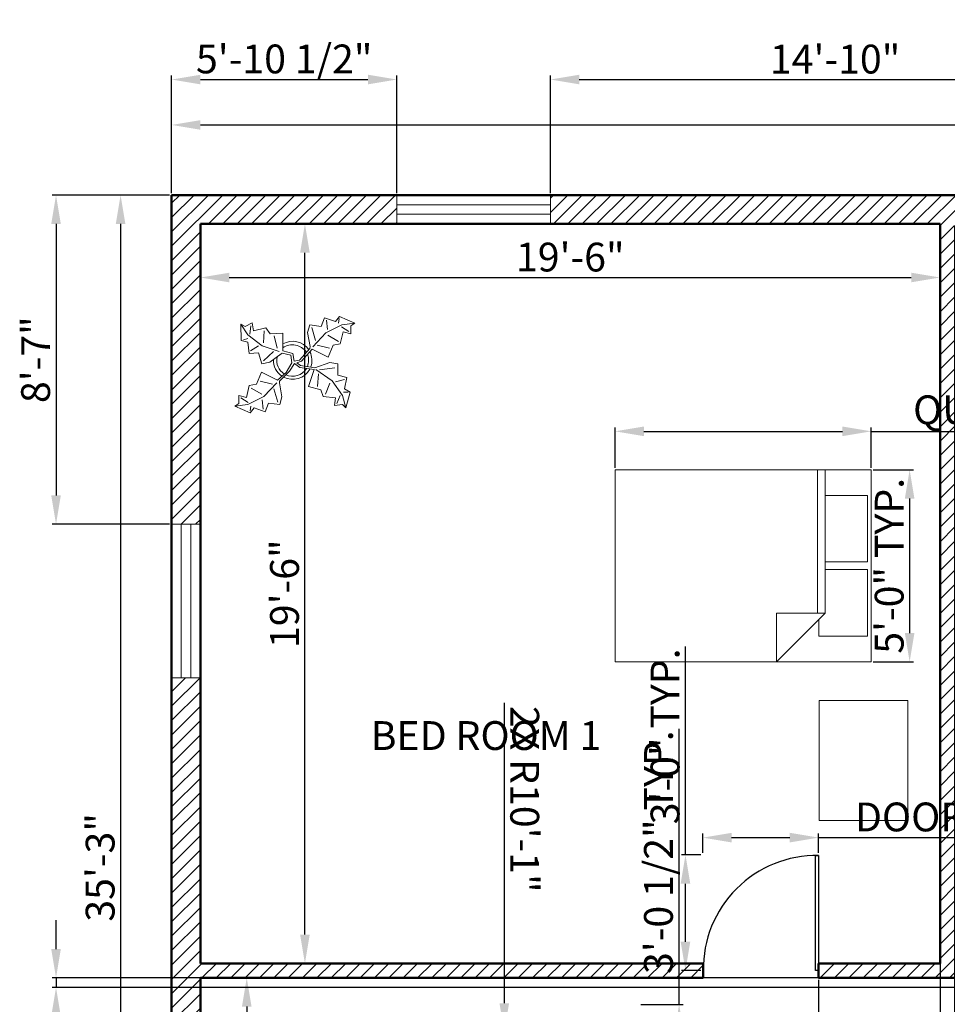
# Model space of a CAD drawing. Units: inches. Extents: x 61993 to 62774, y 55335 to 55871.
# Tile 3 of 6: x 62021 to 62310, y 55563 to 55871. Entities that reach past the tile are written whole.
import ezdxf

# ---------------------------------------------------------------- set-up
doc = ezdxf.new("R2010")
doc.units = ezdxf.units.IN
for name, color, linetype, lineweight in [('A-ANNO-DIMS', 2, 'Continuous', 18), ('A-AREA-IDEN', 7, 'Continuous', 25), ('A-DOOR', 3, 'Continuous', 25), ('A-FURN', 9, 'Continuous', 18), ('A-FURN-PLNT', 94, 'Continuous', 13), ('A-GLAZ', 4, 'Continuous', 18), ('A-WALL', 7, 'Continuous', 50)]:
    doc.layers.add(name, color=color, linetype=linetype, lineweight=lineweight)
doc.layers.add('A-WALL-PATT', color=40, linetype='Continuous', lineweight=13, true_color=0xf8d731)
doc.styles.get("Standard").update_dxf_attribs({"font": 'arial.ttf'})
doc.dimstyles.new('ISO-25', dxfattribs={"dimtxt": 9, "dimasz": 9, "dimexe": 1.25, "dimexo": 0.625, "dimtad": 1, "dimdec": 1, "dimrnd": 9, "dimlunit": 3, "dimtxsty": 'Standard', "dimcen": 2.5, "dimadec": 0, "dimazin": 0, "dimtfac": 1, "dimtdec": 1, "dimtmove": 0, "dimatfit": 3, "dimfxl": 1, "dimarcsym": 0})

# ---------------------------------------------------------------- blocks, each defined once
blk = doc.blocks.new('*D1')
at = {"layer": 'A-ANNO-DIMS', "color": 0, "lineweight": -2, "transparency": 16777216}
for p, q in [((62077.82, 55806.96), (62111.07, 55806.96)), ((62109.82, 55584.96), (62109.82, 55797.96)), ((62077.82, 55575.96), (62111.07, 55575.96))]:
    blk.add_line(p, q, dxfattribs=at)
at = {"layer": 'A-ANNO-DIMS', "color": 0, "transparency": 16777216}
for points in [[(62108.32, 55797.96), (62111.32, 55797.96), (62109.82, 55806.96)], [(62108.32, 55584.96), (62111.32, 55584.96), (62109.82, 55575.96)]]:
    blk.add_solid(points, dxfattribs=at)
at = {"layer": 'Defpoints', "color": 0, "transparency": 16777216}
for p in [(62077.19, 55806.96), (62109.82, 55806.96), (62077.19, 55575.96)]:
    blk.add_point(p, dxfattribs=at)
at = {"layer": 'A-ANNO-DIMS', "color": 0, "transparency": 16777216, "insert": (62104.6, 55691.46), "char_height": 9, "attachment_point": 5, "rotation": 90}
blk.add_mtext('19\'-6"', dxfattribs=at)
blk = doc.blocks.new('*D2')
at = {"layer": 'A-ANNO-DIMS', "color": 0, "lineweight": -2, "transparency": 16777216}
for p, q in [((62077.19, 55806.33), (62077.19, 55788.97)), ((62308.19, 55806.33), (62308.19, 55788.97)), ((62086.19, 55790.22), (62299.19, 55790.22))]:
    blk.add_line(p, q, dxfattribs=at)
at = {"layer": 'A-ANNO-DIMS', "color": 0, "transparency": 16777216}
for points in [[(62086.19, 55791.72), (62086.19, 55788.72), (62077.19, 55790.22)], [(62299.19, 55791.72), (62299.19, 55788.72), (62308.19, 55790.22)]]:
    blk.add_solid(points, dxfattribs=at)
at = {"layer": 'Defpoints', "color": 0, "transparency": 16777216}
for p in [(62077.19, 55806.96), (62308.19, 55806.96), (62308.19, 55790.22)]:
    blk.add_point(p, dxfattribs=at)
at = {"layer": 'A-ANNO-DIMS', "color": 0, "transparency": 16777216, "insert": (62192.69, 55795.44), "char_height": 9, "attachment_point": 5}
blk.add_mtext('19\'-6"', dxfattribs=at)
blk = doc.blocks.new('*D11')
at = {"layer": 'A-ANNO-DIMS', "color": 0, "lineweight": -2, "transparency": 16777216}
for p, q in [((62077.82, 55571.46), (62092.9, 55571.46)), ((62091.65, 55562.46), (62091.65, 55413.96)), ((62077.82, 55404.96), (62092.9, 55404.96))]:
    blk.add_line(p, q, dxfattribs=at)
at = {"layer": 'A-ANNO-DIMS', "color": 0, "transparency": 16777216}
for points in [[(62090.15, 55562.46), (62093.15, 55562.46), (62091.65, 55571.46)], [(62090.15, 55413.96), (62093.15, 55413.96), (62091.65, 55404.96)]]:
    blk.add_solid(points, dxfattribs=at)
at = {"layer": 'Defpoints', "color": 0, "transparency": 16777216}
for p in [(62077.19, 55571.46), (62077.19, 55404.96), (62091.65, 55404.96)]:
    blk.add_point(p, dxfattribs=at)
at = {"layer": 'A-ANNO-DIMS', "color": 0, "transparency": 16777216, "insert": (62086.43, 55488.21), "char_height": 9, "attachment_point": 5, "rotation": 90}
blk.add_mtext('14\'-3"', dxfattribs=at)
blk = doc.blocks.new('Bed - Queen')
for p, q in [((0, -80.00003), (0, 0)), ((0, 0), (59.99999, 0)), ((59.99999, 0), (59.99999, -80.00003)), ((7.99999, -1.2), (28.79998, -1.2)), ((7.99999, -14.4), (7.99999, -1.2)), ((28.79998, -1.2), (28.79998, -14.4)), ((31.19999, -1.2), (51.99999, -1.2)), ((31.19999, -14.4), (31.19999, -1.2)), ((51.99999, -1.2), (51.99999, -16.4)), ((0, -14.4), (44.8, -14.4)), ((59.99999, -29.6), (44.8, -14.4)), ((44.8, -14.4), (44.8, -29.6)), ((44.8, -16.8), (0, -16.8)), ((51.99999, -16.4), (46.79936, -16.4)), ((44.8, -29.6), (59.99999, -29.6)), ((59.99999, -80.00003), (0, -80.00003))]:
    blk.add_line(p, q)
blk = doc.blocks.new('Plant - Rubber or Philodendron')
for p, q in [((8.8871, 10.7908), (9.9809, 13.4933)), ((9.9809, 13.4933), (13.3837, 12.301)), ((10.5828, 12.6946), (10.8893, 9.7953)), ((13.3837, 12.301), (14.68, 13.9039)), ((14.5816, 13.2037), (14.3848, 11.8033)), ((14.68, 13.9039), (19.3848, 11.8146)), ((-16.2005, 11.4774), (-13.9899, 8.1064)), ((-16.2005, 11.4774), (-14.8639, 10.7964)), ((-16.0159, 6.3329), (-16.2005, 11.4774)), ((-14.8639, 10.7964), (-12.6195, 11.8975)), ((-13.3174, 8.325), (-13.0735, 11.0065)), ((-12.6195, 11.8975), (-12.1909, 9.4345)), ((-12.1909, 9.4345), (-8.3829, 10.3)), ((-8.8369, 9.409), (-9.0894, 5.6095)), ((-8.3829, 10.3), (-7.0549, 8.501)), ((4.6914, 8.8812), (5.3859, 11.2828)), ((5.3859, 11.2828), (8.8871, 10.7908)), ((5.9878, 10.4842), (7.1971, 6.3869)), ((15.3859, 11.3055), (10.3916, 8.7942)), ((15.2875, 10.6053), (17.5907, 9.2105)), ((19.3848, 11.8146), (15.3859, 11.3055)), ((19.3848, 11.8146), (18.1868, 10.9119)), ((18.1868, 10.9119), (18.1925, 8.4119)), ((-14.0069, 5.8704), (-16.0159, 6.3329)), ((-15.3434, 6.5514), (-13.9984, 6.9884)), ((-13.9899, 8.1064), (-9.5434, 4.7185)), ((-7.0549, 8.501), (-3.0284, 8.6941)), ((-4.8529, 4.012), (-5.7184, 7.82)), ((-3.0284, 8.6941), (-3.0709, 3.1041)), ((4.6914, 8.8812), (5.5014, 4.4831)), ((10.3916, 8.7942), (6.2847, 4.4028)), ((14.2977, 6.1031), (10.9934, 7.9956)), ((15.7909, 9.1065), (14.8995, 5.3044)), ((18.1925, 8.4119), (15.7909, 9.1065)), ((-13.5868, 2.2894), (-14.0069, 5.8704)), ((-13.1329, 3.1804), (-10.6614, 4.727)), ((-9.5434, 4.7185), (-4.1917, 2.9888)), ((-3.0709, 3.1041), (0.0797, 2.3163)), ((2.1141, 0.2298), (5.4346, 3.9146)), ((6.1032, 3.6844), (2.8262, -0.031)), ((5.4346, 3.9146), (5.5014, 4.4831)), ((11.1089, 1.1958), (6.1032, 3.6844)), ((7.7005, 4.8881), (11.5025, 3.9967)), ((12.7005, 4.8994), (11.1089, 1.1958)), ((14.8995, 5.3044), (12.7005, 4.8994)), ((-10.6784, 2.491), (-13.5868, 2.2894)), ((-9.5858, -0.8715), (-10.6784, 2.491)), ((-9.1318, 0.0195), (-5.9793, 2.9025)), ((-7.1228, -0.443), (-3.5248, 2.2131)), ((-3.5248, 2.2131), (-3.3011, 2.4355)), ((-3.3011, 2.4355), (-0.5306, 1.7947)), ((-0.5306, 1.7947), (-0.2255, -0.5527)), ((-0.5306, 1.7947), (-0.5306, 1.7947)), ((0.0797, 2.3163), (0.4866, -0.031)), ((0.4866, -0.031), (2.1141, 0.2298)), ((-7.1228, -0.443), (-9.5858, -0.8715)), ((-2.019, -3.6148), (-0.2255, -0.5527)), ((-0.9375, -3.1608), (0.5883, -0.8135)), ((0.5883, -0.8135), (2.2447, -2.0916)), ((2.8262, -0.031), (1.3003, -0.5527)), ((1.3003, -0.5527), (2.4193, -1.4655)), ((2.2447, -2.0916), (6.7108, -2.6626)), ((2.4193, -1.4655), (6.895, -2.1175)), ((4.943, -7.9659), (6.7108, -2.6626)), ((11.6605, -0.5413), (6.895, -2.1175)), ((12.3677, -6.1981), (7.219, -2.6772)), ((8.3544, -2.7453), (13.1973, -2.1704)), ((11.6605, -0.5413), (14.1354, -0.8948)), ((14.1354, -0.8948), (14.1354, -4.4304)), ((-11.3237, -7.2629), (-9.7321, -3.5593)), ((-9.7321, -3.5593), (-4.7264, -6.0479)), ((-2.019, -3.6148), (-4.7264, -6.0479)), ((-4.0579, -6.2781), (-0.9375, -3.1608)), ((8.125, -4.0768), (7.7715, -7.9659)), ((16.2567, -5.8446), (13.4283, -6.5517)), ((14.1354, -4.4304), (16.9638, -5.1375)), ((16.9638, -5.1375), (16.2567, -8.673)), ((-14.4141, -11.4699), (-13.5228, -7.6679)), ((-13.5228, -7.6679), (-11.3237, -7.2629)), ((-12.921, -8.4665), (-9.6166, -10.359)), ((-6.3237, -7.2516), (-10.1257, -6.3602)), ((-9.0148, -11.1577), (-4.9047, -6.8122)), ((-4.611, -12.8477), (-5.8203, -8.7504)), ((-4.1246, -6.8466), (-4.0579, -6.2781)), ((-3.3146, -11.2447), (-4.1246, -6.8466)), ((8.8321, -9.0266), (4.943, -7.9659)), ((9.5392, -11.1479), (8.8321, -9.0266)), ((10.2463, -10.4408), (11.6605, -6.9053)), ((15.5496, -10.7943), (12.3677, -6.1981)), ((16.2567, -8.673), (18.0245, -9.7337)), ((-16.8157, -10.7754), (-14.4141, -11.4699)), ((-16.8101, -13.2754), (-16.8157, -10.7754)), ((-13.9107, -12.9688), (-16.2139, -11.574)), ((-14.0091, -13.669), (-9.0148, -11.1577)), ((-9.206, -15.0581), (-9.5126, -12.1588)), ((-3.3146, -11.2447), (-4.0092, -13.6463)), ((13.4283, -11.5015), (9.5392, -11.1479)), ((13.0748, -13.9763), (13.4283, -11.5015)), ((14.8425, -10.7943), (13.7819, -13.2692)), ((16.6103, -14.6834), (15.5496, -10.7943)), ((17.3174, -9.7337), (15.9032, -9.7337)), ((18.0245, -9.7337), (16.6103, -14.6834)), ((-18.008, -14.1781), (-16.8101, -13.2754)), ((-18.008, -14.1781), (-14.0091, -13.669)), ((-13.3032, -16.2674), (-18.008, -14.1781)), ((-12.0069, -14.6645), (-13.3032, -16.2674)), ((-13.2048, -15.5672), (-13.008, -14.1668)), ((-8.6042, -15.8568), (-12.0069, -14.6645)), ((-7.5103, -13.1543), (-8.6042, -15.8568)), ((-4.0092, -13.6463), (-7.5103, -13.1543)), ((15.5496, -13.6228), (13.0748, -13.9763)), ((16.6103, -14.6834), (15.5496, -13.6228))]:
    blk.add_line(p, q)
for centre, radius, start, end in [((0, 0), 6.1275, 34.37569, 120.1028), ((-0.0601, -0.2075), 5.2461, 33.82192, 124.9414), ((0.0308, 0.1664), 6, 178.6147, 235.1169), ((0.0308, 0.1664), 5, 168.1647, 238.6725), ((-0.2664, 0.1682), 5.2775, 338.4094, 20.03007), ((-0.098, 0.1364), 6.1288, 341.2017, 26.09184), ((-0.0234, 0.3825), 6.1492, 242.5812, 331.2714), ((-0.1102, 0.4886), 5.2883, 247.3711, 327.472)]:
    blk.add_arc(centre, radius, start, end)
blk = doc.blocks.new('*D24')
at = {"layer": 'A-ANNO-DIMS', "color": 0, "lineweight": -2, "transparency": 16777216}
for p, q in [((62068.19, 55816.58), (62068.19, 55839.13)), ((62728.19, 55816.58), (62728.19, 55839.13)), ((62077.19, 55837.88), (62719.19, 55837.88))]:
    blk.add_line(p, q, dxfattribs=at)
at = {"layer": 'A-ANNO-DIMS', "color": 0, "transparency": 16777216}
for points in [[(62077.19, 55839.38), (62077.19, 55836.38), (62068.19, 55837.88)], [(62719.19, 55839.38), (62719.19, 55836.38), (62728.19, 55837.88)]]:
    blk.add_solid(points, dxfattribs=at)
at = {"layer": 'Defpoints', "color": 0, "transparency": 16777216}
for p in [(62728.19, 55837.88), (62068.19, 55815.96), (62728.19, 55815.96)]:
    blk.add_point(p, dxfattribs=at)
at = {"layer": 'A-ANNO-DIMS', "color": 0, "transparency": 16777216, "insert": (62398.19, 55843.1), "char_height": 9, "attachment_point": 5}
blk.add_mtext('54\'-9"', dxfattribs=at)
blk = doc.blocks.new('*D27')
at = {"layer": 'A-ANNO-DIMS', "color": 0, "lineweight": -2, "transparency": 16777216}
for p, q in [((62067.57, 55815.96), (62051, 55815.96)), ((62052.25, 55806.96), (62052.25, 55404.96)), ((62067.57, 55395.96), (62051, 55395.96))]:
    blk.add_line(p, q, dxfattribs=at)
at = {"layer": 'A-ANNO-DIMS', "color": 0, "transparency": 16777216}
for points in [[(62050.75, 55806.96), (62053.75, 55806.96), (62052.25, 55815.96)], [(62050.75, 55404.96), (62053.75, 55404.96), (62052.25, 55395.96)]]:
    blk.add_solid(points, dxfattribs=at)
at = {"layer": 'Defpoints', "color": 0, "transparency": 16777216}
for p in [(62068.19, 55815.96), (62052.25, 55395.96), (62068.19, 55395.96)]:
    blk.add_point(p, dxfattribs=at)
at = {"layer": 'A-ANNO-DIMS', "color": 0, "transparency": 16777216, "insert": (62047.03, 55605.96), "char_height": 9, "attachment_point": 5, "rotation": 90}
blk.add_mtext('35\'-3"', dxfattribs=at)
blk = doc.blocks.new('WIN-48IN')
for p, q in [((0, 9), (0, 0)), ((48, 9), (48, 0)), ((48, 6), (0, 6)), ((48, 3), (0, 3))]:
    blk.add_line(p, q)
blk = doc.blocks.new('DOOR-SINGLE-36IN')
for p, q in [((35, 0), (35, 36)), ((35, 36), (36, 36)), ((36, 36), (36, 2.25)), ((36, 0), (35, 0))]:
    blk.add_line(p, q)
blk.add_arc((35.5, 0.5), 35.5, 89.1931, 180.8069)
blk = doc.blocks.new('TABLE-BEDSIDE')
blk.add_lwpolyline([(0, 37.52), (27.74, 37.52), (27.74, 0), (0, 0)], close=True)
blk = doc.blocks.new('*D34')
at = {"layer": 'A-ANNO-DIMS', "color": 0, "lineweight": -2, "transparency": 16777216}
for p, q in [((62234.09, 55610.47), (62234.09, 55616.51)), ((62243.09, 55615.26), (62261.23, 55615.26)), ((62270.23, 55610.47), (62270.23, 55616.51)), ((62270.23, 55615.26), (62376.1, 55615.26))]:
    blk.add_line(p, q, dxfattribs=at)
at = {"layer": 'A-ANNO-DIMS', "color": 0, "transparency": 16777216}
for points in [[(62243.09, 55616.76), (62243.09, 55613.76), (62234.09, 55615.26)], [(62261.23, 55616.76), (62261.23, 55613.76), (62270.23, 55615.26)]]:
    blk.add_solid(points, dxfattribs=at)
at = {"layer": 'Defpoints', "color": 0, "transparency": 16777216}
for p in [(62270.23, 55615.26), (62234.09, 55609.84), (62270.23, 55609.84)]:
    blk.add_point(p, dxfattribs=at)
at = {"layer": 'A-ANNO-DIMS', "color": 0, "transparency": 16777216, "insert": (62327.67, 55620.55), "char_height": 9, "attachment_point": 5}
blk.add_mtext('DOOR 3\'-0" TYP.', dxfattribs=at)
blk = doc.blocks.new('*D35')
at = {"layer": 'A-ANNO-DIMS', "color": 0, "lineweight": -2, "transparency": 16777216}
for p, q in [((62228.67, 55609.84), (62228.67, 55674.94)), ((62233.47, 55609.84), (62227.42, 55609.84)), ((62228.67, 55582.71), (62228.67, 55600.84)), ((62233.47, 55573.71), (62227.42, 55573.71))]:
    blk.add_line(p, q, dxfattribs=at)
at = {"layer": 'A-ANNO-DIMS', "color": 0, "transparency": 16777216}
for points in [[(62227.17, 55600.84), (62230.17, 55600.84), (62228.67, 55609.84)], [(62227.17, 55582.71), (62230.17, 55582.71), (62228.67, 55573.71)]]:
    blk.add_solid(points, dxfattribs=at)
at = {"layer": 'Defpoints', "color": 0, "transparency": 16777216}
for p in [(62228.67, 55609.84), (62234.09, 55609.84), (62234.09, 55573.71)]:
    blk.add_point(p, dxfattribs=at)
at = {"layer": 'A-ANNO-DIMS', "color": 0, "transparency": 16777216, "insert": (62223.45, 55646.89), "char_height": 9, "attachment_point": 5, "rotation": 90}
blk.add_mtext('3\'-0" TYP.', dxfattribs=at)
blk = doc.blocks.new('*D38')
at = {"layer": 'A-ANNO-DIMS', "color": 0, "lineweight": -2, "transparency": 16777216}
for p, q in [((62206.68, 55730.79), (62206.68, 55743.42)), ((62286.68, 55730.79), (62286.68, 55743.42)), ((62215.68, 55742.17), (62277.68, 55742.17)), ((62286.68, 55742.17), (62429.32, 55742.17))]:
    blk.add_line(p, q, dxfattribs=at)
at = {"layer": 'A-ANNO-DIMS', "color": 0, "transparency": 16777216}
for points in [[(62215.68, 55743.67), (62215.68, 55740.67), (62206.68, 55742.17)], [(62277.68, 55743.67), (62277.68, 55740.67), (62286.68, 55742.17)]]:
    blk.add_solid(points, dxfattribs=at)
at = {"layer": 'Defpoints', "color": 0, "transparency": 16777216}
for p in [(62286.68, 55742.17), (62206.68, 55730.17), (62286.68, 55730.17)]:
    blk.add_point(p, dxfattribs=at)
at = {"layer": 'A-ANNO-DIMS', "color": 0, "transparency": 16777216, "insert": (62362.5, 55747.72), "char_height": 9, "attachment_point": 5}
blk.add_mtext('QUEEN BED 6\'-8" TYP.', dxfattribs=at)
blk = doc.blocks.new('*D39')
at = {"layer": 'A-ANNO-DIMS', "color": 0, "lineweight": -2, "transparency": 16777216}
for p, q in [((62287.31, 55730.17), (62299.93, 55730.17)), ((62298.68, 55721.17), (62298.68, 55679.17)), ((62287.31, 55670.17), (62299.93, 55670.17))]:
    blk.add_line(p, q, dxfattribs=at)
at = {"layer": 'A-ANNO-DIMS', "color": 0, "transparency": 16777216}
for points in [[(62297.18, 55721.17), (62300.18, 55721.17), (62298.68, 55730.17)], [(62297.18, 55679.17), (62300.18, 55679.17), (62298.68, 55670.17)]]:
    blk.add_solid(points, dxfattribs=at)
at = {"layer": 'Defpoints', "color": 0, "transparency": 16777216}
for p in [(62286.68, 55730.17), (62286.68, 55670.17), (62298.68, 55670.17)]:
    blk.add_point(p, dxfattribs=at)
at = {"layer": 'A-ANNO-DIMS', "color": 0, "transparency": 16777216, "insert": (62293.46, 55700.17), "char_height": 9, "attachment_point": 5, "rotation": 90}
blk.add_mtext('5\'-0" TYP.', dxfattribs=at)
blk = doc.blocks.new('*D43')
at = {"layer": 'A-ANNO-DIMS', "color": 0, "lineweight": -2, "transparency": 16777216}
for p, q in [((62226.68, 55563.18), (62226.68, 55649.26)), ((62214.71, 55563.18), (62227.93, 55563.18)), ((62226.68, 55535.52), (62226.68, 55554.18)), ((62214.71, 55526.52), (62227.93, 55526.52))]:
    blk.add_line(p, q, dxfattribs=at)
at = {"layer": 'A-ANNO-DIMS', "color": 0, "transparency": 16777216}
for points in [[(62225.18, 55554.18), (62228.18, 55554.18), (62226.68, 55563.18)], [(62225.18, 55535.52), (62228.18, 55535.52), (62226.68, 55526.52)]]:
    blk.add_solid(points, dxfattribs=at)
at = {"layer": 'Defpoints', "color": 0, "transparency": 16777216}
for p in [(62214.08, 55563.18), (62226.68, 55563.18), (62214.08, 55526.52)]:
    blk.add_point(p, dxfattribs=at)
at = {"layer": 'A-ANNO-DIMS', "color": 0, "transparency": 16777216, "insert": (62221.4, 55610.72), "char_height": 9, "attachment_point": 5, "rotation": 90}
blk.add_mtext('3\'-0 1/2" TYP.', dxfattribs=at)
blk = doc.blocks.new('*D64')
at = {"layer": 'A-ANNO-DIMS', "color": 0, "lineweight": -2, "transparency": 16777216}
for p, q in [((62068.19, 55816.58), (62068.19, 55853.31)), ((62077.19, 55852.06), (62129.51, 55852.06)), ((62138.51, 55816.58), (62138.51, 55853.31))]:
    blk.add_line(p, q, dxfattribs=at)
at = {"layer": 'A-ANNO-DIMS', "color": 0, "transparency": 16777216}
for points in [[(62077.19, 55853.56), (62077.19, 55850.56), (62068.19, 55852.06)], [(62129.51, 55853.56), (62129.51, 55850.56), (62138.51, 55852.06)]]:
    blk.add_solid(points, dxfattribs=at)
at = {"layer": 'Defpoints', "color": 0, "transparency": 16777216}
for p in [(62138.51, 55852.06), (62068.19, 55815.96), (62138.51, 55815.96)]:
    blk.add_point(p, dxfattribs=at)
at = {"layer": 'A-ANNO-DIMS', "color": 0, "transparency": 16777216, "insert": (62103.35, 55857.33), "char_height": 9, "attachment_point": 5}
blk.add_mtext('5\'-10 1/2"', dxfattribs=at)
blk = doc.blocks.new('*D65')
at = {"layer": 'A-ANNO-DIMS', "color": 0, "lineweight": -2, "transparency": 16777216}
for p, q in [((62186.51, 55816.58), (62186.51, 55853.31)), ((62195.51, 55852.06), (62355.31, 55852.06)), ((62364.31, 55816.58), (62364.31, 55853.31))]:
    blk.add_line(p, q, dxfattribs=at)
at = {"layer": 'A-ANNO-DIMS', "color": 0, "transparency": 16777216}
for points in [[(62195.51, 55853.56), (62195.51, 55850.56), (62186.51, 55852.06)], [(62355.31, 55853.56), (62355.31, 55850.56), (62364.31, 55852.06)]]:
    blk.add_solid(points, dxfattribs=at)
at = {"layer": 'Defpoints', "color": 0, "transparency": 16777216}
for p in [(62364.31, 55852.06), (62186.51, 55815.96), (62364.31, 55815.96)]:
    blk.add_point(p, dxfattribs=at)
at = {"layer": 'A-ANNO-DIMS', "color": 0, "transparency": 16777216, "insert": (62275.41, 55857.28), "char_height": 9, "attachment_point": 5}
blk.add_mtext('14\'-10"', dxfattribs=at)
blk = doc.blocks.new('*D67')
at = {"layer": 'A-ANNO-DIMS', "color": 0, "lineweight": -2, "transparency": 16777216}
for p, q in [((62067.57, 55815.96), (62030.84, 55815.96)), ((62032.09, 55806.96), (62032.09, 55722.16)), ((62067.57, 55713.16), (62030.84, 55713.16))]:
    blk.add_line(p, q, dxfattribs=at)
at = {"layer": 'A-ANNO-DIMS', "color": 0, "transparency": 16777216}
for points in [[(62030.59, 55806.96), (62033.59, 55806.96), (62032.09, 55815.96)], [(62030.59, 55722.16), (62033.59, 55722.16), (62032.09, 55713.16)]]:
    blk.add_solid(points, dxfattribs=at)
at = {"layer": 'Defpoints', "color": 0, "transparency": 16777216}
for p in [(62068.19, 55815.96), (62032.09, 55713.16), (62068.19, 55713.16)]:
    blk.add_point(p, dxfattribs=at)
at = {"layer": 'A-ANNO-DIMS', "color": 0, "transparency": 16777216, "insert": (62026.87, 55764.56), "char_height": 9, "attachment_point": 5, "rotation": 90}
blk.add_mtext('8\'-7"', dxfattribs=at)
blk = doc.blocks.new('*D71')
at = {"layer": 'A-ANNO-DIMS', "color": 0, "lineweight": -2, "transparency": 16777216}
for p, q in [((62308.19, 55575.33), (62308.19, 55358.61)), ((62270.23, 55570.83), (62270.23, 55358.61)), ((62279.23, 55359.86), (62299.19, 55359.86))]:
    blk.add_line(p, q, dxfattribs=at)
at = {"layer": 'A-ANNO-DIMS', "color": 0, "transparency": 16777216}
for points in [[(62279.23, 55361.36), (62279.23, 55358.36), (62270.23, 55359.86)], [(62299.19, 55361.36), (62299.19, 55358.36), (62308.19, 55359.86)]]:
    blk.add_solid(points, dxfattribs=at)
at = {"layer": 'Defpoints', "color": 0, "transparency": 16777216}
for p in [(62308.19, 55575.96), (62270.23, 55571.46), (62308.19, 55359.86)]:
    blk.add_point(p, dxfattribs=at)
at = {"layer": 'A-ANNO-DIMS', "color": 0, "transparency": 16777216, "insert": (62289.21, 55365.08), "char_height": 9, "attachment_point": 5}
blk.add_mtext('3\'-2"', dxfattribs=at)
blk = doc.blocks.new('*D74')
at = {"layer": 'A-ANNO-DIMS', "color": 0, "lineweight": -2, "transparency": 16777216}
for p, q in [((62032.09, 55580.46), (62032.09, 55589.46)), ((62547.57, 55571.46), (62030.84, 55571.46)), ((62032.09, 55571.46), (62032.09, 55568.46)), ((62547.57, 55568.46), (62030.84, 55568.46)), ((62032.09, 55559.46), (62032.09, 55525.28))]:
    blk.add_line(p, q, dxfattribs=at)
at = {"layer": 'A-ANNO-DIMS', "color": 0, "transparency": 16777216}
for points in [[(62030.59, 55580.46), (62033.59, 55580.46), (62032.09, 55571.46)], [(62030.59, 55559.46), (62033.59, 55559.46), (62032.09, 55568.46)]]:
    blk.add_solid(points, dxfattribs=at)
at = {"layer": 'Defpoints', "color": 0, "transparency": 16777216}
for p in [(62548.19, 55571.46), (62032.09, 55568.46), (62548.19, 55568.46)]:
    blk.add_point(p, dxfattribs=at)
at = {"layer": 'A-ANNO-DIMS', "color": 0, "transparency": 16777216, "insert": (62026.87, 55537.87), "char_height": 9, "attachment_point": 5, "rotation": 90}
blk.add_mtext('0\'-3"', dxfattribs=at)
blk = doc.blocks.new('*D75')
at = {"layer": 'A-ANNO-DIMS', "color": 0, "lineweight": -2, "transparency": 16777216}
for p, q in [((62308.19, 55806.33), (62308.19, 55358.61)), ((62312.69, 55806.33), (62312.69, 55358.61)), ((62299.19, 55359.86), (62290.19, 55359.86)), ((62308.19, 55359.86), (62312.69, 55359.86)), ((62321.69, 55359.86), (62376.84, 55359.86))]:
    blk.add_line(p, q, dxfattribs=at)
at = {"layer": 'A-ANNO-DIMS', "color": 0, "transparency": 16777216}
for points in [[(62299.19, 55361.36), (62299.19, 55358.36), (62308.19, 55359.86)], [(62321.69, 55361.36), (62321.69, 55358.36), (62312.69, 55359.86)]]:
    blk.add_solid(points, dxfattribs=at)
at = {"layer": 'Defpoints', "color": 0, "transparency": 16777216}
for p in [(62308.19, 55806.96), (62312.69, 55806.96), (62312.69, 55359.86)]:
    blk.add_point(p, dxfattribs=at)
at = {"layer": 'A-ANNO-DIMS', "color": 0, "transparency": 16777216, "insert": (62353.77, 55365.13), "char_height": 9, "attachment_point": 5}
blk.add_mtext('0\'-4 1/2"', dxfattribs=at)
blk = doc.blocks.new('*D83')
at = {"layer": 'A-ANNO-DIMS', "color": 0, "lineweight": -2, "transparency": 16777216}
for p, q in [((62172.08, 55657.37), (62172.08, 55563.52)), ((62172.08, 55433.32), (62172.08, 55554.52))]:
    blk.add_line(p, q, dxfattribs=at)
at = {"layer": 'A-ANNO-DIMS', "color": 0, "transparency": 16777216}
blk.add_solid([(62173.58, 55563.52), (62170.58, 55563.52), (62172.08, 55554.52)], dxfattribs=at)
at = {"layer": 'Defpoints', "color": 0, "transparency": 16777216}
for p in [(62172.08, 55554.52), (62172.08, 55433.32)]:
    blk.add_point(p, dxfattribs=at)
at = {"layer": 'A-ANNO-DIMS', "color": 0, "transparency": 16777216, "insert": (62177.3, 55627.24), "char_height": 9, "attachment_point": 5, "rotation": 270.0001}
blk.add_mtext('2X R10\'-1"', dxfattribs=at)

msp = doc.modelspace()

# ---------------------------------------------------------------- hatches: boundary and pattern name
at = {"layer": 'A-WALL-PATT'}
h = msp.add_hatch(dxfattribs=at)
h.set_pattern_fill('ANSI31', color=256)
h.paths.add_polyline_path([(62077.19, 55665.16), (62068.19, 55665.16), (62068.19, 55518.96), (62077.19, 55518.96), (62077.19, 55571.46), (62234.23, 55571.46), (62234.23, 55573.71, -0.007042), (62234.23, 55574.71), (62234.23, 55575.96), (62077.19, 55575.96)])
h.paths.add_polyline_path([(62077.19, 55806.96), (62138.51, 55806.96), (62138.51, 55815.96), (62068.19, 55815.96), (62068.19, 55713.16), (62077.19, 55713.16)])
h.paths.add_polyline_path([(62364.31, 55815.96), (62186.51, 55815.96), (62186.51, 55806.96), (62308.19, 55806.96), (62308.19, 55575.96), (62270.23, 55575.96), (62270.23, 55571.46), (62415.32, 55571.46), (62415.32, 55573.71, -0.007042), (62415.32, 55574.71), (62415.32, 55575.96), (62312.69, 55575.96), (62312.69, 55739.46), (62471.69, 55739.46), (62471.69, 55575.96), (62451.32, 55575.96), (62451.32, 55571.46), (62483.74, 55571.46), (62483.74, 55573.71, -0.007042), (62483.74, 55574.71), (62483.74, 55575.96), (62476.19, 55575.96), (62476.19, 55806.96), (62578.07, 55806.96), (62578.07, 55815.96), (62412.31, 55815.96), (62412.31, 55806.96), (62471.69, 55806.96), (62471.69, 55743.96), (62312.69, 55743.96), (62312.69, 55806.96), (62364.31, 55806.96)])
h.paths.add_polyline_path([(62728.19, 55815.96), (62626.07, 55815.96), (62626.07, 55806.96), (62719.19, 55806.96), (62719.19, 55739.46), (62728.19, 55739.46)])
h.paths.add_polyline_path([(62728.19, 55691.46), (62719.19, 55691.46), (62719.19, 55575.96), (62519.74, 55575.96), (62519.74, 55571.46), (62543.69, 55571.46), (62543.69, 55568.46), (62548.19, 55568.46), (62548.19, 55571.46), (62719.19, 55571.46), (62719.19, 55517.72), (62728.19, 55517.72)])
h.paths.add_polyline_path([(62599.31, 55404.96), (62548.19, 55404.96), (62548.19, 55532.46), (62546.94, 55532.46, -0.007042), (62545.94, 55532.46), (62543.69, 55532.46), (62543.69, 55404.96), (62444.22, 55404.96), (62444.22, 55395.96), (62599.31, 55395.96)])
h.paths.add_polyline_path([(62728.19, 55469.72), (62719.19, 55469.72), (62719.19, 55404.96), (62647.31, 55404.96), (62647.31, 55395.96), (62728.19, 55395.96)])
h.paths.add_polyline_path([(62396.22, 55404.96), (62309.17, 55404.96), (62309.17, 55395.96), (62396.22, 55395.96)])
h.paths.add_polyline_path([(62213.17, 55404.96), (62077.19, 55404.96), (62077.19, 55470.96), (62068.19, 55470.96), (62068.19, 55395.96), (62213.17, 55395.96)])

# ---------------------------------------------------------------- linework, layer by layer
at = {"layer": 'A-WALL'}
for p, q in [((62728.19, 55815.96), (62068.19, 55815.96)), ((62068.19, 55815.96), (62068.19, 55395.96)), ((62077.19, 55806.96), (62077.19, 55575.96)), ((62308.19, 55806.96), (62077.19, 55806.96)), ((62308.19, 55806.96), (62308.19, 55575.96)), ((62234.23, 55575.96), (62077.19, 55575.96)), ((62234.23, 55575.96), (62234.23, 55571.46)), ((62308.19, 55575.96), (62270.23, 55575.96)), ((62270.23, 55575.96), (62270.23, 55571.46)), ((62077.19, 55571.46), (62077.19, 55404.96)), ((62234.23, 55571.46), (62077.19, 55571.46)), ((62415.32, 55571.46), (62270.23, 55571.46))]:
    msp.add_line(p, q, dxfattribs=at)

# ---------------------------------------------------------------- block references
at = {"layer": 'A-DOOR'}
msp.add_blockref('DOOR-SINGLE-36IN', (62234.23, 55573.71), dxfattribs=at)
at = {"layer": 'A-FURN', "rotation": 270}
msp.add_blockref('Bed - Queen', (62286.68, 55730.17), dxfattribs=at)
at = {"layer": 'A-FURN'}
msp.add_blockref('TABLE-BEDSIDE', (62270.38, 55620.59), dxfattribs=at)
at = {"layer": 'A-FURN-PLNT'}
msp.add_blockref('Plant - Rubber or Philodendron', (62105.97, 55764.17), dxfattribs=at)
at = {"layer": 'A-GLAZ'}
msp.add_blockref('WIN-48IN', (62138.51, 55806.96), dxfattribs=at)
at = {"layer": 'A-GLAZ', "rotation": 269.9999999999832}
msp.add_blockref('WIN-48IN', (62068.19, 55713.16), dxfattribs=at)

# ---------------------------------------------------------------- texts
at = {"layer": 'A-AREA-IDEN', "insert": (62130.35, 55651.64), "char_height": 9, "attachment_point": 1}
msp.add_mtext_dynamic_manual_height_columns('BED ROOM 1', width=116.6414, gutter_width=12.5, heights=[0], dxfattribs=at)

# ---------------------------------------------------------------- dimensions: what is measured, and where the dimension line sits
at = {"layer": 'A-ANNO-DIMS'}
for base, p1, p2, override, picture, middle in [((62138.51, 55852.06), (62068.19, 55815.96), (62138.51, 55815.96), {"dimdec": 1, "dimlfac": 1, "dimrnd": 0, "dimzin": 1, "dimdsep": 46, "dimlunit": 4, "dimfrac": 2}, '*D64', (62103.35, 55857.33)), ((62364.31, 55852.06), (62186.51, 55815.96), (62364.31, 55815.96), {"dimdec": 1, "dimlfac": 1, "dimrnd": 0, "dimzin": 1, "dimdsep": 46, "dimlunit": 4, "dimfrac": 2}, '*D65', (62275.41, 55857.28)), ((62728.19, 55837.88), (62068.19, 55815.96), (62728.19, 55815.96), {"dimclrd": 0, "dimclre": 0, "dimclrt": 0}, '*D24', (62398.19, 55843.1)), ((62308.19, 55790.22), (62077.19, 55806.96), (62308.19, 55806.96), {"dimclrd": 0, "dimclre": 0, "dimclrt": 0}, '*D2', (62192.69, 55795.44)), ((62312.69, 55359.86), (62308.19, 55806.96), (62312.69, 55806.96), {"dimdec": 1, "dimlfac": 1, "dimrnd": 0, "dimzin": 1, "dimdsep": 46, "dimlunit": 4, "dimfrac": 2}, '*D75', (62353.77, 55365.13)), ((62308.19, 55359.86), (62270.23, 55571.46), (62308.19, 55575.96), {"dimdec": 1, "dimlfac": 1, "dimrnd": 0, "dimzin": 1, "dimdsep": 46, "dimlunit": 4, "dimfrac": 2}, '*D71', (62289.21, 55365.08))]:
    dim = msp.add_linear_dim(base=base, p1=p1, p2=p2, dimstyle='ISO-25', override=override, dxfattribs=at)
    dim.commit()
    dim.dimension.update_dxf_attribs({"geometry": picture, "text_midpoint": middle})
for base, p1, p2, override, picture, middle in [((62032.09, 55713.16), (62068.19, 55815.96), (62068.19, 55713.16), {"dimdec": 1, "dimlfac": 1, "dimrnd": 0, "dimzin": 1, "dimdsep": 46, "dimlunit": 4, "dimfrac": 2}, '*D67', (62026.87, 55764.56)), ((62052.25, 55395.96), (62068.19, 55815.96), (62068.19, 55395.96), {"dimclrd": 0, "dimclre": 0, "dimclrt": 0}, '*D27', (62047.03, 55605.96)), ((62109.82, 55806.96), (62077.19, 55575.96), (62077.19, 55806.96), {"dimclrd": 0, "dimclre": 0, "dimclrt": 0}, '*D1', (62104.6, 55691.46)), ((62032.09, 55568.46), (62548.19, 55571.46), (62548.19, 55568.46), {"dimdec": 1, "dimlfac": 1, "dimrnd": 0, "dimzin": 1, "dimdsep": 46, "dimlunit": 4, "dimfrac": 2}, '*D74', (62026.87, 55537.87)), ((62091.65, 55404.96), (62077.19, 55571.46), (62077.19, 55404.96), {"dimclrd": 0, "dimclre": 0, "dimclrt": 0}, '*D11', (62086.43, 55488.21))]:
    dim = msp.add_linear_dim(base=base, p1=p1, p2=p2, angle=90, dimstyle='ISO-25', override=override, dxfattribs=at)
    dim.commit()
    dim.dimension.update_dxf_attribs({"geometry": picture, "text_midpoint": middle})
for base, p1, p2, text, picture, middle in [((62286.68, 55742.17), (62206.68, 55730.17), (62286.68, 55730.17), 'QUEEN BED <> TYP.', '*D38', (62362.5, 55747.72)), ((62270.23, 55615.26), (62234.09, 55609.84), (62270.23, 55609.84), 'DOOR <> TYP.', '*D34', (62327.67, 55620.55))]:
    dim = msp.add_linear_dim(base=base, p1=p1, p2=p2, text=text, dimstyle='ISO-25', override={"dimdec": 1, "dimlfac": 1, "dimrnd": 0, "dimzin": 1, "dimdsep": 46, "dimlunit": 4, "dimfrac": 2}, dxfattribs=at)
    dim.commit()
    dim.dimension.update_dxf_attribs({"geometry": picture, "text_midpoint": middle})
for base, p1, p2, angle, picture, middle in [((62298.68, 55670.17), (62286.68, 55730.17), (62286.68, 55670.17), 270, '*D39', (62293.46, 55700.17)), ((62228.67, 55609.84), (62234.09, 55573.71), (62234.09, 55609.84), 90, '*D35', (62223.45, 55646.89)), ((62226.68, 55563.18), (62214.08, 55526.52), (62214.08, 55563.18), 90, '*D43', (62221.4, 55610.72))]:
    dim = msp.add_linear_dim(base=base, p1=p1, p2=p2, angle=angle, text='<> TYP.', dimstyle='ISO-25', override={"dimdec": 1, "dimlfac": 1, "dimrnd": 0, "dimzin": 1, "dimdsep": 46, "dimlunit": 4, "dimfrac": 2}, dxfattribs=at)
    dim.commit()
    dim.dimension.update_dxf_attribs({"geometry": picture, "text_midpoint": middle})
dim = msp.add_radius_dim(center=(62172.08, 55433.32), mpoint=(62172.08, 55554.52), text='2X <>', dimstyle='ISO-25', override={"dimdec": 1, "dimlfac": 1, "dimrnd": 0, "dimzin": 1, "dimdsep": 46, "dimlunit": 4, "dimfrac": 2}, dxfattribs=at)
dim.commit()
dim.dimension.update_dxf_attribs({"geometry": '*D83', "text_midpoint": (62172.08, 55627.24), "dimtype": 164})

doc.saveas('drawing.dxf')
